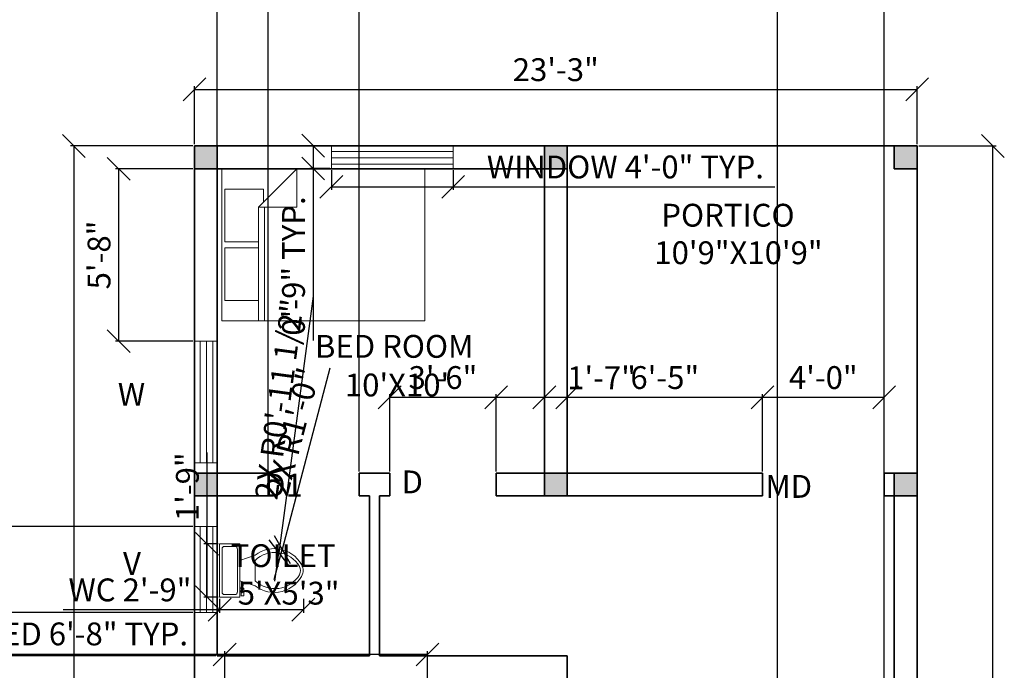
# Model space of a CAD drawing. Units: inches. Extents: x 1798 to 3594, y 1405 to 2404.
# Tile 4 of 6: x 2157 to 2546, y 1789 to 2046. Entities that reach past the tile are written whole.
import ezdxf

# ---------------------------------------------------------------- set-up
doc = ezdxf.new("R2010")
doc.units = ezdxf.units.IN
for name, color, linetype, lineweight in [('A-ANNO-DIMS', 6, 'Continuous', 18), ('A-ANNO-TEXT', 7, 'Continuous', 18), ('A-AREA-IDEN', 242, 'Continuous', 18), ('A-FLOR-FIXT', 242, 'Continuous', 18), ('A-FURN', 18, 'Continuous', 18), ('A-GLAZ', 4, 'Continuous', 18), ('A-WALL', 7, 'Continuous', 35), ('S-COLS', 1, 'Continuous', 35)]:
    doc.layers.add(name, color=color, linetype=linetype, lineweight=lineweight)
doc.styles.get("Standard").update_dxf_attribs({"font": 'arial.ttf'})
doc.dimstyles.new('ISO-25', dxfattribs={"dimtxt": 9, "dimasz": 9, "dimexe": 1.25, "dimexo": 0.625, "dimgap": 2, "dimtad": 1, "dimdec": 1, "dimlunit": 4, "dimtxsty": 'Standard', "dimblk": 'OBLIQUE', "dimcen": 2.5, "dimazin": 0, "dimtfac": 1, "dimtdec": 1, "dimtmove": 0, "dimatfit": 3, "dimfxl": 1, "dimarcsym": 0})

# ---------------------------------------------------------------- blocks, each defined once
blk = doc.blocks.new('_Oblique')
at = {"color": 0, "linetype": 'ByBlock', "lineweight": -2}
blk.add_line((-0.5, -0.5), (0.5, 0.5), dxfattribs=at)
blk = doc.blocks.new('*D2')
at = {"layer": 'A-ANNO-DIMS', "color": 0, "lineweight": -2, "transparency": 16777216}
for p, q in [((2226.27, 1996.44), (2226.27, 2019.35)), ((2226.27, 2018.1), (2511.27, 2018.1)), ((2511.27, 1996.44), (2511.27, 2019.35))]:
    blk.add_line(p, q, dxfattribs=at)
at = {"layer": 'Defpoints', "color": 0, "transparency": 16777216}
for p in [(2511.27, 2018.1), (2226.27, 1995.81), (2511.27, 1995.81)]:
    blk.add_point(p, dxfattribs=at)
at = {"layer": 'A-ANNO-DIMS', "color": 0, "lineweight": -2, "transparency": 16777216, "xscale": 9, "yscale": 9, "zscale": 9, "rotation": 180}
blk.add_blockref('_Oblique', (2226.27, 2018.1), dxfattribs=at)
at = {"layer": 'A-ANNO-DIMS', "color": 0, "lineweight": -2, "transparency": 16777216, "xscale": 9, "yscale": 9, "zscale": 9}
blk.add_blockref('_Oblique', (2511.27, 2018.1), dxfattribs=at)
at = {"layer": 'A-ANNO-DIMS', "color": 0, "transparency": 16777216, "insert": (2368.77, 2024.7), "char_height": 9, "attachment_point": 5}
blk.add_mtext('23\'-3"', dxfattribs=at)
blk = doc.blocks.new('*D3')
at = {"layer": 'A-ANNO-DIMS', "color": 0, "lineweight": -2, "transparency": 16777216}
for p, q in [((2225.65, 1995.81), (2177.4, 1995.81)), ((2178.65, 1995.81), (2178.65, 1551.81)), ((2225.65, 1551.81), (2177.4, 1551.81))]:
    blk.add_line(p, q, dxfattribs=at)
at = {"layer": 'Defpoints', "color": 0, "transparency": 16777216}
for p in [(2226.27, 1995.81), (2178.65, 1551.81), (2226.27, 1551.81)]:
    blk.add_point(p, dxfattribs=at)
at = {"layer": 'A-ANNO-DIMS', "color": 0, "lineweight": -2, "transparency": 16777216, "xscale": 9, "yscale": 9, "zscale": 9}
for p, rotation in [((2178.65, 1995.81), 90), ((2178.65, 1551.81), 270)]:
    blk.add_blockref('_Oblique', p, dxfattribs=dict(at, rotation=rotation))
at = {"layer": 'A-ANNO-DIMS', "color": 0, "transparency": 16777216, "insert": (2172.06, 1773.81), "char_height": 9, "attachment_point": 5, "rotation": 90}
blk.add_mtext("37'", dxfattribs=at)
blk = doc.blocks.new('Toilet - top')
for p, q in [((9.5, -6), (9.5, -2)), ((-10, -8.5), (-8, -8.5)), ((-10, -9.5), (-10, -8.5)), ((-7, -9.5), (-10, -9.5)), ((-8, -8.5), (-8, -8)), ((-7, -8), (-7, -9.5)), ((-4, -8), (-6, -14)), ((4, -8), (6, -14)), ((4, -14), (-4, -14))]:
    blk.add_line(p, q)
blk.add_lwpolyline([(10.5, -8), (10.5, 0), (-10.5, 0), (-10.5, -8)], close=True)
for points in [[(-9.5, -2), (-9.5, -6)], [(8.5, -1), (-8.5, -1)], [(-8.5, -7), (8.5, -7)]]:
    blk.add_lwpolyline(points)
for centre, radius, start, end in [((-8.62, -1.88), 0.884, 81.8699, 188.1301), ((8.62, -1.88), 0.884, 351.8699, 98.1301), ((-8.62, -6.12), 0.884, 171.8699, 278.1301), ((8.62, -6.12), 0.884, 261.8699, 8.1301), ((3.52, -21.58), 12.17, 141.4691, 247.9714), ((4.2, -21.82), 11.33, 136.3677, 238.9468), ((-3.52, -21.58), 12.17, 292.0284, 38.5307), ((-4.2, -21.82), 11.33, 301.053, 43.6321), ((0, -27.88), 4, 245.7318, 294.2682), ((0, -29), 4, 254.8605, 285.1395)]:
    blk.add_arc(centre, radius, start, end)
blk = doc.blocks.new('Bed - Queen')
for p, q in [((0, -80.00003), (0, 0)), ((0, 0), (59.99999, 0)), ((59.99999, 0), (59.99999, -80.00003)), ((7.99999, -1.2), (28.79998, -1.2)), ((7.99999, -14.4), (7.99999, -1.2)), ((28.79998, -1.2), (28.79998, -14.4)), ((31.19999, -1.2), (51.99999, -1.2)), ((31.19999, -14.4), (31.19999, -1.2)), ((51.99999, -1.2), (51.99999, -16.4)), ((0, -14.4), (44.8, -14.4)), ((59.99999, -29.6), (44.8, -14.4)), ((44.8, -14.4), (44.8, -29.6)), ((44.8, -16.8), (0, -16.8)), ((51.99999, -16.4), (46.79936, -16.4)), ((44.8, -29.6), (59.99999, -29.6)), ((59.99999, -80.00003), (0, -80.00003))]:
    blk.add_line(p, q)
blk = doc.blocks.new('COLUMN-9X9')
h = blk.add_hatch(color=256)
h.dxf.hatch_style = 1
h.paths.add_polyline_path([(9, 9), (0, 9), (0, 0), (9, 0)])
blk.add_lwpolyline([(0, 9), (9, 9), (9, 0), (0, 0)], close=True)
blk = doc.blocks.new('WINDOW-48-PLAN')
for p, q in [((0, 48), (9, 48)), ((2.25, 48), (2.25, 0)), ((4.75, 48), (4.75, 0)), ((7.25, 48), (7.25, 0)), ((7.25, 48), (7.25, 0)), ((0, 0), (9, 0))]:
    blk.add_line(p, q)
blk = doc.blocks.new('*D17')
at = {"layer": 'A-ANNO-DIMS', "color": 0, "lineweight": -2, "transparency": 16777216}
for p, q in [((2280.27, 1986.27), (2280.27, 1978.45)), ((2328.27, 1986.27), (2328.27, 1978.45)), ((2280.27, 1979.7), (2328.27, 1979.7)), ((2328.27, 1979.7), (2455.16, 1979.7))]:
    blk.add_line(p, q, dxfattribs=at)
at = {"layer": 'Defpoints', "color": 0, "transparency": 16777216}
for p in [(2280.27, 1986.9), (2328.27, 1986.9), (2328.27, 1979.7)]:
    blk.add_point(p, dxfattribs=at)
at = {"layer": 'A-ANNO-DIMS', "color": 0, "lineweight": -2, "transparency": 16777216, "xscale": 9, "yscale": 9, "zscale": 9, "rotation": 180}
blk.add_blockref('_Oblique', (2280.27, 1979.7), dxfattribs=at)
at = {"layer": 'A-ANNO-DIMS', "color": 0, "lineweight": -2, "transparency": 16777216, "xscale": 9, "yscale": 9, "zscale": 9}
blk.add_blockref('_Oblique', (2328.27, 1979.7), dxfattribs=at)
at = {"layer": 'A-ANNO-DIMS', "color": 0, "transparency": 16777216, "insert": (2396.21, 1986.35), "char_height": 9, "attachment_point": 5}
blk.add_mtext('WINDOW 4\'-0" TYP.', dxfattribs=at)
blk = doc.blocks.new('*D18')
at = {"layer": 'A-ANNO-DIMS', "color": 0, "lineweight": -2, "transparency": 16777216}
for p, q in [((2279.65, 1995.9), (2271.82, 1995.9)), ((2273.07, 1995.9), (2273.07, 1986.9)), ((2279.65, 1986.9), (2271.82, 1986.9)), ((2273.07, 1986.9), (2273.07, 1919.04))]:
    blk.add_line(p, q, dxfattribs=at)
at = {"layer": 'Defpoints', "color": 0, "transparency": 16777216}
for p in [(2280.27, 1995.9), (2273.07, 1986.9), (2280.27, 1986.9)]:
    blk.add_point(p, dxfattribs=at)
at = {"layer": 'A-ANNO-DIMS', "color": 0, "lineweight": -2, "transparency": 16777216, "xscale": 9, "yscale": 9, "zscale": 9}
for p, rotation in [((2273.07, 1995.9), 90), ((2273.07, 1986.9), 270)]:
    blk.add_blockref('_Oblique', p, dxfattribs=dict(at, rotation=rotation))
at = {"layer": 'A-ANNO-DIMS', "color": 0, "transparency": 16777216, "insert": (2266.48, 1948.47), "char_height": 9, "attachment_point": 5, "rotation": 90}
blk.add_mtext('0\'-9" TYP.', dxfattribs=at)
blk = doc.blocks.new('*D19')
at = {"layer": 'A-ANNO-DIMS', "color": 0, "lineweight": -2, "transparency": 16777216}
for p, q in [((2238.18, 1795.31), (2092.79, 1795.31)), ((2238.18, 1783.93), (2238.18, 1796.56)), ((2318.18, 1795.31), (2238.18, 1795.31)), ((2318.18, 1783.93), (2318.18, 1796.56))]:
    blk.add_line(p, q, dxfattribs=at)
at = {"layer": 'Defpoints', "color": 0, "transparency": 16777216}
for p in [(2238.18, 1795.31), (2238.18, 1783.31), (2318.18, 1783.31)]:
    blk.add_point(p, dxfattribs=at)
at = {"layer": 'A-ANNO-DIMS', "color": 0, "lineweight": -2, "transparency": 16777216, "xscale": 9, "yscale": 9, "zscale": 9, "rotation": 180}
blk.add_blockref('_Oblique', (2238.18, 1795.31), dxfattribs=at)
at = {"layer": 'A-ANNO-DIMS', "color": 0, "lineweight": -2, "transparency": 16777216, "xscale": 9, "yscale": 9, "zscale": 9}
blk.add_blockref('_Oblique', (2318.18, 1795.31), dxfattribs=at)
at = {"layer": 'A-ANNO-DIMS', "color": 0, "transparency": 16777216, "insert": (2160.99, 1802.24), "char_height": 9, "attachment_point": 5}
blk.add_mtext('QUEEN BED 6\'-8" TYP.', dxfattribs=at)
blk = doc.blocks.new('*D23')
at = {"layer": 'A-ANNO-DIMS', "color": 0, "lineweight": -2, "transparency": 16777216}
for p, q in [((2236.17, 1817.28), (2236.17, 1811.69)), ((2269.22, 1817.28), (2269.22, 1811.69)), ((2236.17, 1812.94), (2174.44, 1812.94)), ((2269.22, 1812.94), (2236.17, 1812.94))]:
    blk.add_line(p, q, dxfattribs=at)
at = {"layer": 'Defpoints', "color": 0, "transparency": 16777216}
for p in [(2236.17, 1817.9), (2269.22, 1817.9), (2236.17, 1812.94)]:
    blk.add_point(p, dxfattribs=at)
at = {"layer": 'A-ANNO-DIMS', "color": 0, "lineweight": -2, "transparency": 16777216, "xscale": 9, "yscale": 9, "zscale": 9, "rotation": 180}
blk.add_blockref('_Oblique', (2236.17, 1812.94), dxfattribs=at)
at = {"layer": 'A-ANNO-DIMS', "color": 0, "lineweight": -2, "transparency": 16777216, "xscale": 9, "yscale": 9, "zscale": 9}
blk.add_blockref('_Oblique', (2269.22, 1812.94), dxfattribs=at)
at = {"layer": 'A-ANNO-DIMS', "color": 0, "transparency": 16777216, "insert": (2200.81, 1819.6), "char_height": 9, "attachment_point": 5}
blk.add_mtext('WC 2\'-9"', dxfattribs=at)
blk = doc.blocks.new('*D24')
at = {"layer": 'A-ANNO-DIMS', "color": 0, "lineweight": -2, "transparency": 16777216}
for p, q in [((2231.22, 1838.9), (2231.22, 1874.98)), ((2235.55, 1838.9), (2229.97, 1838.9)), ((2231.22, 1817.9), (2231.22, 1838.9)), ((2235.55, 1817.9), (2229.97, 1817.9))]:
    blk.add_line(p, q, dxfattribs=at)
at = {"layer": 'Defpoints', "color": 0, "transparency": 16777216}
for p in [(2231.22, 1838.9), (2236.17, 1838.9), (2236.17, 1817.9)]:
    blk.add_point(p, dxfattribs=at)
at = {"layer": 'A-ANNO-DIMS', "color": 0, "lineweight": -2, "transparency": 16777216, "xscale": 9, "yscale": 9, "zscale": 9}
for p, rotation in [((2231.22, 1838.9), 90), ((2231.22, 1817.9), 270)]:
    blk.add_blockref('_Oblique', p, dxfattribs=dict(at, rotation=rotation))
at = {"layer": 'A-ANNO-DIMS', "color": 0, "transparency": 16777216, "insert": (2224.62, 1861.44), "char_height": 9, "attachment_point": 5, "rotation": 90}
blk.add_mtext('1\'-9"', dxfattribs=at)
blk = doc.blocks.new('*D30')
at = {"layer": 'A-ANNO-DIMS', "color": 0, "lineweight": -2, "transparency": 16777216}
for p, q in [((2511.9, 1995.81), (2542.42, 1995.81)), ((2541.17, 1479.81), (2541.17, 1995.81)), ((2342.9, 1479.81), (2542.42, 1479.81))]:
    blk.add_line(p, q, dxfattribs=at)
at = {"layer": 'Defpoints', "color": 0, "transparency": 16777216}
for p in [(2511.27, 1995.81), (2541.17, 1995.81), (2342.27, 1479.81)]:
    blk.add_point(p, dxfattribs=at)
at = {"layer": 'A-ANNO-DIMS', "color": 0, "lineweight": -2, "transparency": 16777216, "xscale": 9, "yscale": 9, "zscale": 9}
for p, rotation in [((2541.17, 1995.81), 90), ((2541.17, 1479.81), 270)]:
    blk.add_blockref('_Oblique', p, dxfattribs=dict(at, rotation=rotation))
at = {"layer": 'A-ANNO-DIMS', "color": 0, "transparency": 16777216, "insert": (2534.57, 1737.81), "char_height": 9, "attachment_point": 5, "rotation": 90}
blk.add_mtext('43\'-0"', dxfattribs=at)
blk = doc.blocks.new('*D34')
at = {"layer": 'A-ANNO-DIMS', "color": 0, "lineweight": -2, "transparency": 16777216}
for p, q in [((2303.27, 1867.44), (2303.27, 1897.96)), ((2303.27, 1896.71), (2345.27, 1896.71)), ((2345.27, 1867.44), (2345.27, 1897.96))]:
    blk.add_line(p, q, dxfattribs=at)
at = {"layer": 'Defpoints', "color": 0, "transparency": 16777216}
for p in [(2345.27, 1896.71), (2303.27, 1866.81), (2345.27, 1866.81)]:
    blk.add_point(p, dxfattribs=at)
at = {"layer": 'A-ANNO-DIMS', "color": 0, "lineweight": -2, "transparency": 16777216, "xscale": 9, "yscale": 9, "zscale": 9, "rotation": 180}
blk.add_blockref('_Oblique', (2303.27, 1896.71), dxfattribs=at)
at = {"layer": 'A-ANNO-DIMS', "color": 0, "lineweight": -2, "transparency": 16777216, "xscale": 9, "yscale": 9, "zscale": 9}
blk.add_blockref('_Oblique', (2345.27, 1896.71), dxfattribs=at)
at = {"layer": 'A-ANNO-DIMS', "color": 0, "transparency": 16777216, "insert": (2324.27, 1903.31), "char_height": 9, "attachment_point": 5}
blk.add_mtext('3\'-6"', dxfattribs=at)
blk = doc.blocks.new('*D35')
at = {"layer": 'A-ANNO-DIMS', "color": 0, "lineweight": -2, "transparency": 16777216}
for p, q in [((2345.27, 1867.44), (2345.27, 1897.96)), ((2345.27, 1896.71), (2364.27, 1896.71)), ((2364.27, 1867.44), (2364.27, 1897.96)), ((2364.27, 1896.71), (2400.35, 1896.71))]:
    blk.add_line(p, q, dxfattribs=at)
at = {"layer": 'Defpoints', "color": 0, "transparency": 16777216}
for p in [(2364.27, 1896.71), (2345.27, 1866.81), (2364.27, 1866.81)]:
    blk.add_point(p, dxfattribs=at)
at = {"layer": 'A-ANNO-DIMS', "color": 0, "lineweight": -2, "transparency": 16777216, "xscale": 9, "yscale": 9, "zscale": 9, "rotation": 180}
blk.add_blockref('_Oblique', (2345.27, 1896.71), dxfattribs=at)
at = {"layer": 'A-ANNO-DIMS', "color": 0, "lineweight": -2, "transparency": 16777216, "xscale": 9, "yscale": 9, "zscale": 9}
blk.add_blockref('_Oblique', (2364.27, 1896.71), dxfattribs=at)
at = {"layer": 'A-ANNO-DIMS', "color": 0, "transparency": 16777216, "insert": (2386.81, 1903.23), "char_height": 9, "attachment_point": 5}
blk.add_mtext('1\'-7"', dxfattribs=at)
blk = doc.blocks.new('*D36')
at = {"layer": 'A-ANNO-DIMS', "color": 0, "lineweight": -2, "transparency": 16777216}
for p, q in [((2373.27, 1867.44), (2373.27, 1897.96)), ((2373.27, 1896.71), (2450.27, 1896.71)), ((2450.27, 1867.44), (2450.27, 1897.96))]:
    blk.add_line(p, q, dxfattribs=at)
at = {"layer": 'Defpoints', "color": 0, "transparency": 16777216}
for p in [(2450.27, 1896.71), (2373.27, 1866.81), (2450.27, 1866.81)]:
    blk.add_point(p, dxfattribs=at)
at = {"layer": 'A-ANNO-DIMS', "color": 0, "lineweight": -2, "transparency": 16777216, "xscale": 9, "yscale": 9, "zscale": 9, "rotation": 180}
blk.add_blockref('_Oblique', (2373.27, 1896.71), dxfattribs=at)
at = {"layer": 'A-ANNO-DIMS', "color": 0, "lineweight": -2, "transparency": 16777216, "xscale": 9, "yscale": 9, "zscale": 9}
blk.add_blockref('_Oblique', (2450.27, 1896.71), dxfattribs=at)
at = {"layer": 'A-ANNO-DIMS', "color": 0, "transparency": 16777216, "insert": (2411.77, 1903.31), "char_height": 9, "attachment_point": 5}
blk.add_mtext('6\'-5"', dxfattribs=at)
blk = doc.blocks.new('*D37')
at = {"layer": 'A-ANNO-DIMS', "color": 0, "lineweight": -2, "transparency": 16777216}
for p, q in [((2450.27, 1867.44), (2450.27, 1897.96)), ((2450.27, 1896.71), (2498.27, 1896.71)), ((2498.27, 1867.44), (2498.27, 1897.96))]:
    blk.add_line(p, q, dxfattribs=at)
at = {"layer": 'Defpoints', "color": 0, "transparency": 16777216}
for p in [(2498.27, 1896.71), (2450.27, 1866.81), (2498.27, 1866.81)]:
    blk.add_point(p, dxfattribs=at)
at = {"layer": 'A-ANNO-DIMS', "color": 0, "lineweight": -2, "transparency": 16777216, "xscale": 9, "yscale": 9, "zscale": 9, "rotation": 180}
blk.add_blockref('_Oblique', (2450.27, 1896.71), dxfattribs=at)
at = {"layer": 'A-ANNO-DIMS', "color": 0, "lineweight": -2, "transparency": 16777216, "xscale": 9, "yscale": 9, "zscale": 9}
blk.add_blockref('_Oblique', (2498.27, 1896.71), dxfattribs=at)
at = {"layer": 'A-ANNO-DIMS', "color": 0, "transparency": 16777216, "insert": (2474.27, 1903.31), "char_height": 9, "attachment_point": 5}
blk.add_mtext('4\'-0"', dxfattribs=at)
blk = doc.blocks.new('*D40')
at = {"layer": 'A-ANNO-DIMS', "color": 0, "lineweight": -2, "transparency": 16777216}
for p, q in [((2225.65, 1986.81), (2195.12, 1986.81)), ((2196.37, 1918.81), (2196.37, 1986.81)), ((2225.65, 1918.81), (2195.12, 1918.81))]:
    blk.add_line(p, q, dxfattribs=at)
at = {"layer": 'Defpoints', "color": 0, "transparency": 16777216}
for p in [(2196.37, 1986.81), (2226.27, 1986.81), (2226.27, 1918.81)]:
    blk.add_point(p, dxfattribs=at)
at = {"layer": 'A-ANNO-DIMS', "color": 0, "lineweight": -2, "transparency": 16777216, "xscale": 9, "yscale": 9, "zscale": 9}
for p, rotation in [((2196.37, 1986.81), 90), ((2196.37, 1918.81), 270)]:
    blk.add_blockref('_Oblique', p, dxfattribs=dict(at, rotation=rotation))
at = {"layer": 'A-ANNO-DIMS', "color": 0, "transparency": 16777216, "insert": (2189.78, 1952.81), "char_height": 9, "attachment_point": 5, "rotation": 90}
blk.add_mtext('5\'-8"', dxfattribs=at)
blk = doc.blocks.new('*D42')
at = {"layer": 'A-ANNO-DIMS', "color": 0, "lineweight": -2, "transparency": 16777216}
for p, q in [((2235.27, 1867.44), (2235.27, 2092.43)), ((2235.27, 2091.18), (2255.27, 2091.18)), ((2255.27, 1867.44), (2255.27, 2092.43)), ((2255.27, 2091.18), (2291.35, 2091.18))]:
    blk.add_line(p, q, dxfattribs=at)
at = {"layer": 'Defpoints', "color": 0, "transparency": 16777216}
for p in [(2255.27, 2091.18), (2235.27, 1866.81), (2255.27, 1866.81)]:
    blk.add_point(p, dxfattribs=at)
at = {"layer": 'A-ANNO-DIMS', "color": 0, "lineweight": -2, "transparency": 16777216, "xscale": 9, "yscale": 9, "zscale": 9, "rotation": 180}
blk.add_blockref('_Oblique', (2235.27, 2091.18), dxfattribs=at)
at = {"layer": 'A-ANNO-DIMS', "color": 0, "lineweight": -2, "transparency": 16777216, "xscale": 9, "yscale": 9, "zscale": 9}
blk.add_blockref('_Oblique', (2255.27, 2091.18), dxfattribs=at)
at = {"layer": 'A-ANNO-DIMS', "color": 0, "transparency": 16777216, "insert": (2277.81, 2097.78), "char_height": 9, "attachment_point": 5}
blk.add_mtext('1\'-8"', dxfattribs=at)
blk = doc.blocks.new('*D43')
at = {"layer": 'A-ANNO-DIMS', "color": 0, "lineweight": -2, "transparency": 16777216}
for p, q in [((2255.27, 1867.44), (2255.27, 2092.43)), ((2255.27, 2091.18), (2291.27, 2091.18)), ((2291.27, 1867.44), (2291.27, 2092.43))]:
    blk.add_line(p, q, dxfattribs=at)
at = {"layer": 'Defpoints', "color": 0, "transparency": 16777216}
for p in [(2291.27, 2091.18), (2255.27, 1866.81), (2291.27, 1866.81)]:
    blk.add_point(p, dxfattribs=at)
at = {"layer": 'A-ANNO-DIMS', "color": 0, "lineweight": -2, "transparency": 16777216, "xscale": 9, "yscale": 9, "zscale": 9, "rotation": 180}
blk.add_blockref('_Oblique', (2255.27, 2091.18), dxfattribs=at)
at = {"layer": 'A-ANNO-DIMS', "color": 0, "lineweight": -2, "transparency": 16777216, "xscale": 9, "yscale": 9, "zscale": 9}
blk.add_blockref('_Oblique', (2291.27, 2091.18), dxfattribs=at)
at = {"layer": 'A-ANNO-DIMS', "color": 0, "transparency": 16777216, "insert": (2273.27, 2097.78), "char_height": 9, "attachment_point": 5}
blk.add_mtext('3\'-0"', dxfattribs=at)
blk = doc.blocks.new('*D44')
at = {"layer": 'A-ANNO-DIMS', "color": 0, "lineweight": -2, "transparency": 16777216}
for p, q in [((2037.37, 1845.81), (2037.37, 1889.88)), ((2225.65, 1845.81), (2036.12, 1845.81)), ((2037.37, 1811.81), (2037.37, 1845.81)), ((2225.65, 1811.81), (2036.12, 1811.81))]:
    blk.add_line(p, q, dxfattribs=at)
at = {"layer": 'Defpoints', "color": 0, "transparency": 16777216}
for p in [(2037.37, 1845.81), (2226.27, 1845.81), (2226.27, 1811.81)]:
    blk.add_point(p, dxfattribs=at)
at = {"layer": 'A-ANNO-DIMS', "color": 0, "lineweight": -2, "transparency": 16777216, "xscale": 9, "yscale": 9, "zscale": 9}
for p, rotation in [((2037.37, 1845.81), 90), ((2037.37, 1811.81), 270)]:
    blk.add_blockref('_Oblique', p, dxfattribs=dict(at, rotation=rotation))
at = {"layer": 'A-ANNO-DIMS', "color": 0, "transparency": 16777216, "insert": (2030.78, 1872.35), "char_height": 9, "attachment_point": 5, "rotation": 90}
blk.add_mtext('2\'-10"', dxfattribs=at)
blk = doc.blocks.new('*D45')
at = {"layer": 'A-ANNO-DIMS', "color": 0, "lineweight": -2, "transparency": 16777216}
for p, q in [((2037.37, 1811.81), (2037.37, 1847.89)), ((2225.65, 1811.81), (2036.12, 1811.81)), ((2037.37, 1794.81), (2037.37, 1811.81)), ((2234.65, 1794.81), (2036.12, 1794.81))]:
    blk.add_line(p, q, dxfattribs=at)
at = {"layer": 'Defpoints', "color": 0, "transparency": 16777216}
for p in [(2037.37, 1811.81), (2226.27, 1811.81), (2235.27, 1794.81)]:
    blk.add_point(p, dxfattribs=at)
at = {"layer": 'A-ANNO-DIMS', "color": 0, "lineweight": -2, "transparency": 16777216, "xscale": 9, "yscale": 9, "zscale": 9}
for p, rotation in [((2037.37, 1811.81), 90), ((2037.37, 1794.81), 270)]:
    blk.add_blockref('_Oblique', p, dxfattribs=dict(at, rotation=rotation))
at = {"layer": 'A-ANNO-DIMS', "color": 0, "transparency": 16777216, "insert": (2030.78, 1834.35), "char_height": 9, "attachment_point": 5, "rotation": 90}
blk.add_mtext('1\'-5"', dxfattribs=at)
blk = doc.blocks.new('*D47')
at = {"layer": 'A-ANNO-DIMS', "color": 0, "lineweight": -2, "transparency": 16777216}
for p, q in [((2456.27, 1666.44), (2456.27, 2092.43)), ((2456.27, 2091.18), (2498.27, 2091.18)), ((2498.27, 1666.44), (2498.27, 2092.43))]:
    blk.add_line(p, q, dxfattribs=at)
at = {"layer": 'Defpoints', "color": 0, "transparency": 16777216}
for p in [(2498.27, 2091.18), (2456.27, 1665.81), (2498.27, 1665.81)]:
    blk.add_point(p, dxfattribs=at)
at = {"layer": 'A-ANNO-DIMS', "color": 0, "lineweight": -2, "transparency": 16777216, "xscale": 9, "yscale": 9, "zscale": 9, "rotation": 180}
blk.add_blockref('_Oblique', (2456.27, 2091.18), dxfattribs=at)
at = {"layer": 'A-ANNO-DIMS', "color": 0, "lineweight": -2, "transparency": 16777216, "xscale": 9, "yscale": 9, "zscale": 9}
blk.add_blockref('_Oblique', (2498.27, 2091.18), dxfattribs=at)
at = {"layer": 'A-ANNO-DIMS', "color": 0, "transparency": 16777216, "insert": (2477.27, 2097.78), "char_height": 9, "attachment_point": 5}
blk.add_mtext('3\'-6"', dxfattribs=at)
blk = doc.blocks.new('*D79')
at = {"layer": 'A-ANNO-DIMS', "color": 0, "lineweight": -2, "transparency": 16777216}
for p in [(2279.66, 1908.25), (2257.75, 1824.88)]:
    blk.add_line(p, (2260.84, 1836.65), dxfattribs=at)
at = {"layer": 'Defpoints', "color": 0, "transparency": 16777216}
for p in [(2260.84, 1836.65), (2257.75, 1824.88)]:
    blk.add_point(p, dxfattribs=at)
at = {"layer": 'A-ANNO-DIMS', "color": 0, "lineweight": -2, "transparency": 16777216, "xscale": 9, "yscale": 9, "zscale": 9, "rotation": 255.2794917317179}
blk.add_blockref('_Oblique', (2260.84, 1836.65), dxfattribs=at)
at = {"layer": 'A-ANNO-DIMS', "color": 0, "transparency": 16777216, "insert": (2266.16, 1882.83), "char_height": 9, "attachment_point": 5, "rotation": 75.2795}
blk.add_mtext('2X R1\'-0"', dxfattribs=at)
blk = doc.blocks.new('*D80')
at = {"layer": 'A-ANNO-DIMS', "color": 0, "lineweight": -2, "transparency": 16777216}
for p in [(2273.09, 1936.51), (2257.99, 1824.2)]:
    blk.add_line(p, (2259.5, 1835.43), dxfattribs=at)
at = {"layer": 'Defpoints', "color": 0, "transparency": 16777216}
for p in [(2259.5, 1835.43), (2257.99, 1824.2)]:
    blk.add_point(p, dxfattribs=at)
at = {"layer": 'A-ANNO-DIMS', "color": 0, "lineweight": -2, "transparency": 16777216, "xscale": 9, "yscale": 9, "zscale": 9, "rotation": 262.3437976901704}
blk.add_blockref('_Oblique', (2259.5, 1835.43), dxfattribs=at)
at = {"layer": 'A-ANNO-DIMS', "color": 0, "transparency": 16777216, "insert": (2260.9, 1895.78), "char_height": 9, "attachment_point": 5, "rotation": 82.3438}
blk.add_mtext('2X R0\'-11 1/2"', dxfattribs=at)

msp = doc.modelspace()

# ---------------------------------------------------------------- linework, layer by layer
at = {"layer": 'A-GLAZ'}
for p, q in [((2226.27, 1845.81), (2235.27, 1845.81)), ((2228.52, 1845.81), (2228.52, 1811.81)), ((2231.02, 1845.81), (2231.02, 1811.81)), ((2233.52, 1845.81), (2233.52, 1811.81)), ((2233.52, 1845.81), (2233.52, 1811.81)), ((2226.27, 1811.81), (2235.27, 1811.81))]:
    msp.add_line(p, q, dxfattribs=at)
at = {"layer": 'A-WALL'}
for p, q in [((2226.27, 1995.81), (2511.27, 1995.81)), ((2226.27, 1995.81), (2226.27, 1551.81)), ((2364.27, 1995.81), (2364.27, 1857.81)), ((2373.27, 1995.81), (2373.27, 1857.81)), ((2511.27, 1995.81), (2511.27, 1551.81)), ((2235.27, 1986.81), (2373.27, 1986.81)), ((2235.27, 1986.81), (2235.27, 1794.81)), ((2226.27, 1866.81), (2255.27, 1866.81)), ((2255.27, 1866.81), (2255.27, 1857.81)), ((2291.27, 1866.81), (2291.27, 1857.81)), ((2291.27, 1866.81), (2303.27, 1866.81)), ((2303.27, 1866.81), (2303.27, 1857.81)), ((2345.27, 1866.81), (2345.27, 1857.81)), ((2345.27, 1866.81), (2364.27, 1866.81)), ((2373.27, 1866.81), (2450.27, 1866.81)), ((2450.27, 1866.81), (2450.27, 1857.81)), ((2498.27, 1866.81), (2498.27, 1857.81)), ((2498.27, 1866.81), (2511.27, 1866.81)), ((2226.27, 1857.81), (2255.27, 1857.81)), ((2291.27, 1857.81), (2295.27, 1857.81)), ((2295.27, 1857.81), (2295.27, 1794.81)), ((2299.27, 1857.81), (2299.27, 1794.81)), ((2299.27, 1857.81), (2303.27, 1857.81)), ((2345.27, 1857.81), (2450.27, 1857.81)), ((2498.27, 1857.81), (2511.27, 1857.81)), ((2502.27, 1857.81), (2502.27, 1551.81)), ((2235.27, 1794.81), (2295.27, 1794.81)), ((2299.27, 1794.81), (2373.27, 1794.81)), ((2373.27, 1794.81), (2373.27, 1717.81))]:
    msp.add_line(p, q, dxfattribs=at)

# ---------------------------------------------------------------- block references
at = {"layer": 'A-FLOR-FIXT', "rotation": 90}
msp.add_blockref('Toilet - top', (2236.17, 1828.4), dxfattribs=at)
at = {"layer": 'A-FURN', "rotation": 90}
msp.add_blockref('Bed - Queen', (2237.06, 1926.81), dxfattribs=at)
at = {"layer": 'A-GLAZ', "rotation": 270.0000000000011}
msp.add_blockref('WINDOW-48-PLAN', (2280.27, 1995.9), dxfattribs=at)
at = {"layer": 'A-GLAZ'}
msp.add_blockref('WINDOW-48-PLAN', (2226.27, 1870.81), dxfattribs=at)
at = {"layer": 'S-COLS'}
for p in [(2226.27, 1986.81), (2364.27, 1986.81), (2502.27, 1986.81), (2226.27, 1857.81), (2364.27, 1857.81), (2502.27, 1857.81)]:
    msp.add_blockref('COLUMN-9X9', p, dxfattribs=at)

# ---------------------------------------------------------------- texts
at = {"layer": 'A-ANNO-TEXT'}
for s, p in [('               W', (2154.77, 1893.39)), ('              D1', (2215.21, 1857.57)), ('               D', (2266.68, 1858.84)), ('              MD', (2412.93, 1857.06)), ('                V', (2154.08, 1826.66))]:
    msp.add_text(s, height=9, dxfattribs=at).set_placement(p)
at = {"layer": 'A-AREA-IDEN'}
for s, p in [('  PORTICO', (2404.88, 1963.99)), (' 10\'9"X10\'9"', (2404.88, 1949.2)), ('BED ROOM', (2273.77, 1912.28)), ("   10'X10'", (2277.34, 1897.05)), ('  TOILET', (2235.08, 1829.76)), ('   5\'X5\'3"', (2235.08, 1814.97))]:
    msp.add_text(s, height=9, dxfattribs=at).set_placement(p)

# ---------------------------------------------------------------- dimensions: what is measured, and where the dimension line sits
at = {"layer": 'A-ANNO-DIMS'}
for base, p1, p2, picture, middle in [((2255.27, 2091.18), (2235.27, 1866.81), (2255.27, 1866.81), '*D42', (2277.81, 2097.78)), ((2291.27, 2091.18), (2255.27, 1866.81), (2291.27, 1866.81), '*D43', (2273.27, 2097.78)), ((2498.27, 2091.18), (2456.27, 1665.81), (2498.27, 1665.81), '*D47', (2477.27, 2097.78)), ((2345.27, 1896.71), (2303.27, 1866.81), (2345.27, 1866.81), '*D34', (2324.27, 1903.31)), ((2364.27, 1896.71), (2345.27, 1866.81), (2364.27, 1866.81), '*D35', (2386.81, 1903.23)), ((2450.27, 1896.71), (2373.27, 1866.81), (2450.27, 1866.81), '*D36', (2411.77, 1903.31)), ((2498.27, 1896.71), (2450.27, 1866.81), (2498.27, 1866.81), '*D37', (2474.27, 1903.31))]:
    dim = msp.add_linear_dim(base=base, p1=p1, p2=p2, dimstyle='ISO-25', override={"dimdec": 1, "dimlfac": 1, "dimrnd": 0, "dimzin": 1, "dimdsep": 46, "dimlunit": 4, "dimfrac": 2}, dxfattribs=at)
    dim.commit()
    dim.dimension.update_dxf_attribs({"geometry": picture, "text_midpoint": middle})
dim = msp.add_linear_dim(base=(2511.27, 2018.1), p1=(2226.27, 1995.81), p2=(2511.27, 1995.81), text='23\'-3"', dimstyle='ISO-25', override={"dimclrd": 0, "dimclre": 0, "dimclrt": 0}, dxfattribs=at)
dim.commit()
dim.dimension.update_dxf_attribs({"geometry": '*D2', "text_midpoint": (2368.77, 2024.7)})
for base, p1, p2, angle, text, picture, middle in [((2328.27, 1979.7), (2280.27, 1986.9), (2328.27, 1986.9), 0, 'WINDOW <> TYP.', '*D17', (2396.21, 1986.35)), ((2273.07, 1986.9), (2280.27, 1995.9), (2280.27, 1986.9), 270, '<> TYP.', '*D18', (2266.48, 1948.47)), ((2236.1722, 1812.9445), (2269.2185, 1817.9014), (2236.1722, 1817.9014), 180, 'WC <>', '*D23', (2200.8059, 1819.598)), ((2238.18, 1795.31), (2318.18, 1783.31), (2238.18, 1783.31), 180, 'QUEEN BED <> TYP.', '*D19', (2160.99, 1802.24))]:
    dim = msp.add_linear_dim(base=base, p1=p1, p2=p2, angle=angle, text=text, dimstyle='ISO-25', override={"dimdec": 1, "dimlfac": 1, "dimrnd": 0, "dimzin": 1, "dimdsep": 46, "dimlunit": 4, "dimfrac": 2}, dxfattribs=at)
    dim.commit()
    dim.dimension.update_dxf_attribs({"geometry": picture, "text_midpoint": middle})
for base, p1, p2, override, picture, middle in [((2178.65, 1551.81), (2226.27, 1995.81), (2226.27, 1551.81), {"dimclrd": 0, "dimclre": 0, "dimclrt": 0}, '*D3', (2172.06, 1773.81)), ((2541.17, 1995.81), (2342.27, 1479.81), (2511.27, 1995.81), {"dimdec": 1, "dimlfac": 1, "dimrnd": 0, "dimzin": 1, "dimdsep": 46, "dimlunit": 4, "dimfrac": 2}, '*D30', (2534.57, 1737.81)), ((2196.37, 1986.81), (2226.27, 1918.81), (2226.27, 1986.81), {"dimdec": 1, "dimlfac": 1, "dimrnd": 0, "dimzin": 1, "dimdsep": 46, "dimlunit": 4, "dimfrac": 2}, '*D40', (2189.78, 1952.81)), ((2037.37, 1845.81), (2226.27, 1811.81), (2226.27, 1845.81), {"dimdec": 1, "dimlfac": 1, "dimrnd": 0, "dimzin": 1, "dimdsep": 46, "dimlunit": 4, "dimfrac": 2}, '*D44', (2030.78, 1872.35)), ((2231.22, 1838.9), (2236.17, 1817.9), (2236.17, 1838.9), {"dimdec": 1, "dimlfac": 1, "dimrnd": 0, "dimzin": 1, "dimdsep": 46, "dimlunit": 4, "dimfrac": 2}, '*D24', (2224.62, 1861.44)), ((2037.37, 1811.81), (2235.27, 1794.81), (2226.27, 1811.81), {"dimdec": 1, "dimlfac": 1, "dimrnd": 0, "dimzin": 1, "dimdsep": 46, "dimlunit": 4, "dimfrac": 2}, '*D45', (2030.78, 1834.35))]:
    dim = msp.add_linear_dim(base=base, p1=p1, p2=p2, angle=90, dimstyle='ISO-25', override=override, dxfattribs=at)
    dim.commit()
    dim.dimension.update_dxf_attribs({"geometry": picture, "text_midpoint": middle})
for center, mpoint, picture, middle in [((2257.99, 1824.2), (2259.5, 1835.43), '*D80', (2260.9, 1895.78)), ((2257.75, 1824.88), (2260.84, 1836.65), '*D79', (2266.16, 1882.83))]:
    dim = msp.add_radius_dim(center=center, mpoint=mpoint, text='2X <>', dimstyle='ISO-25', override={"dimdec": 1, "dimlfac": 1, "dimrnd": 0, "dimzin": 1, "dimdsep": 46, "dimlunit": 4, "dimfrac": 2}, dxfattribs=at)
    dim.commit()
    dim.dimension.update_dxf_attribs({"geometry": picture, "text_midpoint": middle})

doc.saveas('drawing.dxf')
